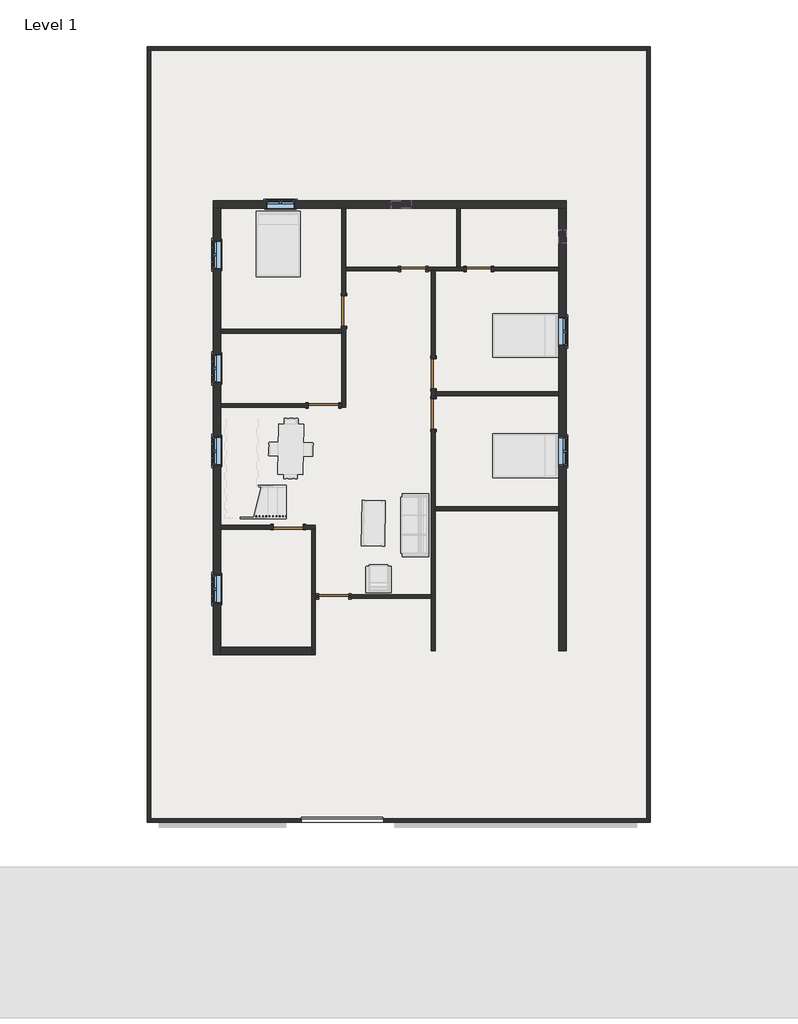
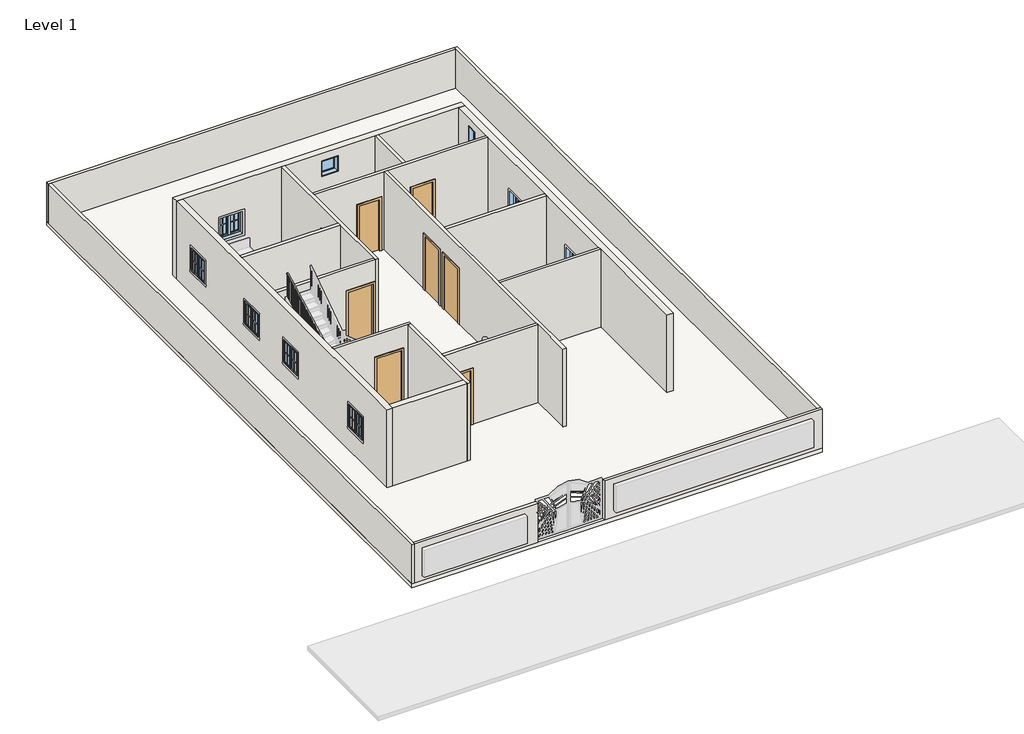
# One storey, part 1 of 2: 20 walls, 9 windows, 8 doors, 1 railing, 1 slab.
"""IFC4 building model written with IfcOpenShell, lengths in millimetres."""

from ifc_helpers import new_model, si_unit, frame, origin, origin_with_axes, place, context, project, spatial, polyline, outline, extrude, faceted_brep, transform, mapped, element, save
from components import door_d8f5dbb5, door_f2b275c1, door_305aa2a5, door_e5f9f3c4, window_aa618e30, window_80340324, window_339605e1

model = new_model("IFC4")

# Units and contexts
model_context = context("Model", 3, world=origin())
ifc_project = project(units=[si_unit("LENGTHUNIT", "METRE", prefix="MILLI")], contexts=[model_context])

# Site, building, storey
site = spatial("IfcSite", under=ifc_project)
building = spatial("IfcBuilding", under=site)
storey = spatial("IfcBuildingStorey", under=building, Name="Level 1", Elevation=0.0)

# Doors
placement = place(None, origin())
door_shape = door_d8f5dbb5(model_context)
element("IfcDoor", 1, ObjectType="Single-Flush : 30\" x 80\"", at=placement, inside=storey, context=model_context, shape_type="MappedRepresentation", body=[
    mapped(door_shape, transform((-551.6099931, 5332.4435985, 0.0), x_axis=(1.0, 0.0, 0.0), y_axis=(0.0, 1.0, 0.0), z_axis=(0.0, 0.0, 1.0))),
])
door_2_shape = door_f2b275c1(model_context)
element("IfcDoor", 2, ObjectType="Single-Flush : 30\" x 80\"", at=placement, inside=storey, context=model_context, shape_type="MappedRepresentation", body=[
    mapped(door_2_shape, transform((1429.5900069, 5332.4435985, 0.0), x_axis=(-1.0, 0.0, 0.0), y_axis=(0.0, -1.0, 0.0), z_axis=(0.0, 0.0, 1.0))),
])
door_3_shape = door_305aa2a5(model_context)
element("IfcDoor", 3, ObjectType="Single-Flush : 36\" x 84\"", at=placement, inside=storey, context=model_context, shape_type="MappedRepresentation", body=[
    mapped(door_3_shape, transform((-2647.1099931, 4062.4435985, 0.0), x_axis=(0.0, -1.0, 0.0), y_axis=(1.0, 0.0, 0.0), z_axis=(0.0, 0.0, 1.0))),
])
element("IfcDoor", 4, ObjectType="Single-Flush : 36\" x 84\"", at=placement, inside=storey, context=model_context, shape_type="MappedRepresentation", body=[
    mapped(door_3_shape, transform((57.9900069, 2170.1435985, 0.0), x_axis=(0.0, -1.0, 0.0), y_axis=(1.0, 0.0, 0.0), z_axis=(0.0, 0.0, 1.0))),
])
element("IfcDoor", 5, ObjectType="Single-Flush : 36\" x 84\"", at=placement, inside=storey, context=model_context, shape_type="MappedRepresentation", body=[
    mapped(door_3_shape, transform((-4323.5099931, -2465.3564015, 0.0), x_axis=(1.0, 0.0, 0.0), y_axis=(0.0, 1.0, 0.0), z_axis=(0.0, 0.0, 1.0))),
])
element("IfcDoor", 6, ObjectType="Single-Flush : 36\" x 84\"", at=placement, inside=storey, context=model_context, shape_type="MappedRepresentation", body=[
    mapped(door_3_shape, transform((-2951.9099931, -4560.8564015, 0.0), x_axis=(-1.0, 0.0, 0.0), y_axis=(0.0, -1.0, 0.0), z_axis=(0.0, 0.0, 1.0))),
])
door_4_shape = door_e5f9f3c4(model_context)
element("IfcDoor", 7, ObjectType="Single-Flush : 36\" x 84\"", at=placement, inside=storey, context=model_context, shape_type="MappedRepresentation", body=[
    mapped(door_4_shape, transform((-3256.7099931, 1204.9435985, 0.0), x_axis=(1.0, 0.0, 0.0), y_axis=(0.0, 1.0, 0.0), z_axis=(0.0, 0.0, 1.0))),
])
element("IfcDoor", 8, ObjectType="Single-Flush : 36\" x 84\"", at=placement, inside=storey, context=model_context, shape_type="MappedRepresentation", body=[
    mapped(door_4_shape, transform((57.9900069, 950.9435985, 0.0), x_axis=(0.0, 1.0, 0.0), y_axis=(-1.0, 0.0, 0.0), z_axis=(0.0, 0.0, 1.0))),
])

# Railing
element("IfcRailing", 9, ObjectType="Handrail - Rectangular", at=placement, inside=storey, context=model_context, shape_type="SolidModel", body=[
    faceted_brep([(-4378.4230036, -2160.5564015, 1761.0666667), (-4378.4230036, -2160.5564015, 1704.9107192), (-4378.4230036, -2109.7564015, 1704.9107192), (-4378.4230036, -2109.7564015, 1761.0666667), (-5973.5005957, -2160.5564015, 2512.5835228), (-5984.8684735, -2160.5564015, 2461.7835228), (-5984.8684735, -2109.7564015, 2461.7835228), (-5973.5005957, -2109.7564015, 2512.5835228), (-6196.7599931, -2160.5564015, 2512.5835228), (-6196.7599931, -2160.5564015, 2461.7835228), (-6145.9599931, -2109.7564015, 2461.7835228), (-6145.9599931, -2109.7564015, 2512.5835228), (-6196.7599931, -1959.3194067, 2512.5835228), (-6196.7599931, -1946.6862419, 2461.7835228), (-6145.9599931, -1946.6862419, 2461.7835228), (-6145.9599931, -1959.3194067, 2512.5835228), (-6196.7599931, 775.380588, 3962.4), (-6145.9599931, 775.380588, 3962.4), (-6145.9599931, 775.380588, 3904.9024571), (-6196.7599931, 775.380588, 3904.9024571)], [[[0, 1, 2, 3]], [[1, 0, 4, 5]], [[2, 1, 5, 6]], [[3, 2, 6, 7]], [[0, 3, 7, 4]], [[5, 4, 8, 9]], [[6, 5, 9, 10]], [[7, 6, 10, 11]], [[4, 7, 11, 8]], [[9, 8, 12, 13]], [[10, 9, 13, 14]], [[11, 10, 14, 15]], [[8, 11, 15, 12]], [[16, 17, 18, 19]], [[13, 12, 16, 19]], [[14, 13, 19, 18]], [[15, 14, 18, 17]], [[12, 15, 17, 16]]]),
    extrude(outline(polyline([(719.1685985, 3875.1013569), (719.1685985, 2878.6666667), (700.1185985, 2878.6666667), (700.1185985, 3865.001893), (719.1685985, 3875.1013569)])), frame((-6180.8849931, 0.0, 0.0), z_axis=(1.0, 0.0, 0.0), x_axis=(0.0, 1.0, 0.0)), (0.0, 0.0, 1.0), 19.05),
    extrude(outline(polyline([(617.5685985, 3821.2375494), (617.5685985, 2878.6666667), (598.5185985, 2878.6666667), (598.5185985, 3811.1380855), (617.5685985, 3821.2375494)])), frame((-6180.8849931, 0.0, 0.0), z_axis=(1.0, 0.0, 0.0), x_axis=(0.0, 1.0, 0.0)), (0.0, 0.0, 1.0), 19.05),
    extrude(outline(polyline([(515.9685985, 3767.3737419), (515.9685985, 2878.6666667), (496.9185985, 2878.6666667), (496.9185985, 3757.274278), (515.9685985, 3767.3737419)])), frame((-6180.8849931, 0.0, 0.0), z_axis=(1.0, 0.0, 0.0), x_axis=(0.0, 1.0, 0.0)), (0.0, 0.0, 1.0), 19.05),
    extrude(outline(polyline([(414.3685985, 3713.5099344), (414.3685985, 2709.3333333), (395.3185985, 2709.3333333), (395.3185985, 3703.4104705), (414.3685985, 3713.5099344)])), frame((-6180.8849931, 0.0, 0.0), z_axis=(1.0, 0.0, 0.0), x_axis=(0.0, 1.0, 0.0)), (0.0, 0.0, 1.0), 19.05),
    extrude(outline(polyline([(312.7685985, 3659.6461269), (312.7685985, 2709.3333333), (293.7185985, 2709.3333333), (293.7185985, 3649.546663), (312.7685985, 3659.6461269)])), frame((-6180.8849931, 0.0, 0.0), z_axis=(1.0, 0.0, 0.0), x_axis=(0.0, 1.0, 0.0)), (0.0, 0.0, 1.0), 19.05),
    extrude(outline(polyline([(211.1685985, 3605.7823194), (211.1685985, 2540.0), (192.1185985, 2540.0), (192.1185985, 3595.6828555), (211.1685985, 3605.7823194)])), frame((-6180.8849931, 0.0, 0.0), z_axis=(1.0, 0.0, 0.0), x_axis=(0.0, 1.0, 0.0)), (0.0, 0.0, 1.0), 19.05),
    extrude(outline(polyline([(109.5685985, 3551.9185119), (109.5685985, 2540.0), (90.5185985, 2540.0), (90.5185985, 3541.819048), (109.5685985, 3551.9185119)])), frame((-6180.8849931, 0.0, 0.0), z_axis=(1.0, 0.0, 0.0), x_axis=(0.0, 1.0, 0.0)), (0.0, 0.0, 1.0), 19.05),
    extrude(outline(polyline([(7.9685985, 3498.0547044), (7.9685985, 2540.0), (-11.0814015, 2540.0), (-11.0814015, 3487.9552405), (7.9685985, 3498.0547044)])), frame((-6180.8849931, 0.0, 0.0), z_axis=(1.0, 0.0, 0.0), x_axis=(0.0, 1.0, 0.0)), (0.0, 0.0, 1.0), 19.05),
    extrude(outline(polyline([(-93.6314015, 3444.1908969), (-93.6314015, 2370.6666667), (-112.6814015, 2370.6666667), (-112.6814015, 3434.091433), (-93.6314015, 3444.1908969)])), frame((-6180.8849931, 0.0, 0.0), z_axis=(1.0, 0.0, 0.0), x_axis=(0.0, 1.0, 0.0)), (0.0, 0.0, 1.0), 19.05),
    extrude(outline(polyline([(-195.2314015, 3390.3270894), (-195.2314015, 2370.6666667), (-214.2814015, 2370.6666667), (-214.2814015, 3380.2276255), (-195.2314015, 3390.3270894)])), frame((-6180.8849931, 0.0, 0.0), z_axis=(1.0, 0.0, 0.0), x_axis=(0.0, 1.0, 0.0)), (0.0, 0.0, 1.0), 19.05),
    extrude(outline(polyline([(-296.8314015, 3336.4632819), (-296.8314015, 2370.6666667), (-315.8814015, 2370.6666667), (-315.8814015, 3326.363818), (-296.8314015, 3336.4632819)])), frame((-6180.8849931, 0.0, 0.0), z_axis=(1.0, 0.0, 0.0), x_axis=(0.0, 1.0, 0.0)), (0.0, 0.0, 1.0), 19.05),
    extrude(outline(polyline([(-398.4314015, 3282.5994744), (-398.4314015, 2201.3333333), (-417.4814015, 2201.3333333), (-417.4814015, 3272.5000105), (-398.4314015, 3282.5994744)])), frame((-6180.8849931, 0.0, 0.0), z_axis=(1.0, 0.0, 0.0), x_axis=(0.0, 1.0, 0.0)), (0.0, 0.0, 1.0), 19.05),
    extrude(outline(polyline([(-500.0314015, 3228.7356669), (-500.0314015, 2201.3333333), (-519.0814015, 2201.3333333), (-519.0814015, 3218.636203), (-500.0314015, 3228.7356669)])), frame((-6180.8849931, 0.0, 0.0), z_axis=(1.0, 0.0, 0.0), x_axis=(0.0, 1.0, 0.0)), (0.0, 0.0, 1.0), 19.05),
    extrude(outline(polyline([(-601.6314015, 3174.8718594), (-601.6314015, 2201.3333333), (-620.6814015, 2201.3333333), (-620.6814015, 3164.7723955), (-601.6314015, 3174.8718594)])), frame((-6180.8849931, 0.0, 0.0), z_axis=(1.0, 0.0, 0.0), x_axis=(0.0, 1.0, 0.0)), (0.0, 0.0, 1.0), 19.05),
    extrude(outline(polyline([(-703.2314015, 3121.0080519), (-703.2314015, 2032.0), (-722.2814015, 2032.0), (-722.2814015, 3110.908588), (-703.2314015, 3121.0080519)])), frame((-6180.8849931, 0.0, 0.0), z_axis=(1.0, 0.0, 0.0), x_axis=(0.0, 1.0, 0.0)), (0.0, 0.0, 1.0), 19.05),
    extrude(outline(polyline([(-804.8314015, 3067.1442444), (-804.8314015, 2032.0), (-823.8814015, 2032.0), (-823.8814015, 3057.0447805), (-804.8314015, 3067.1442444)])), frame((-6180.8849931, 0.0, 0.0), z_axis=(1.0, 0.0, 0.0), x_axis=(0.0, 1.0, 0.0)), (0.0, 0.0, 1.0), 19.05),
    extrude(outline(polyline([(-906.4314015, 3013.2804369), (-906.4314015, 2032.0), (-925.4814015, 2032.0), (-925.4814015, 3003.180973), (-906.4314015, 3013.2804369)])), frame((-6180.8849931, 0.0, 0.0), z_axis=(1.0, 0.0, 0.0), x_axis=(0.0, 1.0, 0.0)), (0.0, 0.0, 1.0), 19.05),
    extrude(outline(polyline([(-1008.0314015, 2959.4166294), (-1008.0314015, 1862.6666667), (-1027.0814015, 1862.6666667), (-1027.0814015, 2949.3171655), (-1008.0314015, 2959.4166294)])), frame((-6180.8849931, 0.0, 0.0), z_axis=(1.0, 0.0, 0.0), x_axis=(0.0, 1.0, 0.0)), (0.0, 0.0, 1.0), 19.05),
    extrude(outline(polyline([(-1109.6314015, 2905.5528219), (-1109.6314015, 1862.6666667), (-1128.6814015, 1862.6666667), (-1128.6814015, 2895.453358), (-1109.6314015, 2905.5528219)])), frame((-6180.8849931, 0.0, 0.0), z_axis=(1.0, 0.0, 0.0), x_axis=(0.0, 1.0, 0.0)), (0.0, 0.0, 1.0), 19.05),
    extrude(outline(polyline([(-1211.2314015, 2851.6890144), (-1211.2314015, 1862.6666667), (-1230.2814015, 1862.6666667), (-1230.2814015, 2841.5895505), (-1211.2314015, 2851.6890144)])), frame((-6180.8849931, 0.0, 0.0), z_axis=(1.0, 0.0, 0.0), x_axis=(0.0, 1.0, 0.0)), (0.0, 0.0, 1.0), 19.05),
    extrude(outline(polyline([(-1312.8314015, 2797.8252069), (-1312.8314015, 1862.6666667), (-1331.8814015, 1862.6666667), (-1331.8814015, 2787.725743), (-1312.8314015, 2797.8252069)])), frame((-6180.8849931, 0.0, 0.0), z_axis=(1.0, 0.0, 0.0), x_axis=(0.0, 1.0, 0.0)), (0.0, 0.0, 1.0), 19.05),
    extrude(outline(polyline([(-1414.4314015, 2743.9613994), (-1414.4314015, 1693.3333333), (-1433.4814015, 1693.3333333), (-1433.4814015, 2733.8619355), (-1414.4314015, 2743.9613994)])), frame((-6180.8849931, 0.0, 0.0), z_axis=(1.0, 0.0, 0.0), x_axis=(0.0, 1.0, 0.0)), (0.0, 0.0, 1.0), 19.05),
    extrude(outline(polyline([(-1516.0314015, 2690.0975919), (-1516.0314015, 1693.3333333), (-1535.0814015, 1693.3333333), (-1535.0814015, 2679.998128), (-1516.0314015, 2690.0975919)])), frame((-6180.8849931, 0.0, 0.0), z_axis=(1.0, 0.0, 0.0), x_axis=(0.0, 1.0, 0.0)), (0.0, 0.0, 1.0), 19.05),
    extrude(outline(polyline([(-1617.6314015, 2636.2337844), (-1617.6314015, 1693.3333333), (-1636.6814015, 1693.3333333), (-1636.6814015, 2626.1343205), (-1617.6314015, 2636.2337844)])), frame((-6180.8849931, 0.0, 0.0), z_axis=(1.0, 0.0, 0.0), x_axis=(0.0, 1.0, 0.0)), (0.0, 0.0, 1.0), 19.05),
    extrude(outline(polyline([(-1719.2314015, 2582.3699769), (-1719.2314015, 1693.3333333), (-1738.2814015, 1693.3333333), (-1738.2814015, 2572.270513), (-1719.2314015, 2582.3699769)])), frame((-6180.8849931, 0.0, 0.0), z_axis=(1.0, 0.0, 0.0), x_axis=(0.0, 1.0, 0.0)), (0.0, 0.0, 1.0), 19.05),
    extrude(outline(polyline([(-1820.8314015, 2528.5061694), (-1820.8314015, 1524.0), (-1839.8814015, 1524.0), (-1839.8814015, 2518.4067055), (-1820.8314015, 2528.5061694)])), frame((-6180.8849931, 0.0, 0.0), z_axis=(1.0, 0.0, 0.0), x_axis=(0.0, 1.0, 0.0)), (0.0, 0.0, 1.0), 19.05),
    extrude(outline(polyline([(-1922.4314015, 2474.6423619), (-1922.4314015, 1524.0), (-1941.4814015, 1524.0), (-1941.4814015, 2464.542898), (-1922.4314015, 2474.6423619)])), frame((-6180.8849931, 0.0, 0.0), z_axis=(1.0, 0.0, 0.0), x_axis=(0.0, 1.0, 0.0)), (0.0, 0.0, 1.0), 19.05),
    extrude(outline(polyline([(-6180.8849931, -2043.0814015), (-6180.8849931, -2024.0314015), (-6161.8349931, -2024.0314015), (-6161.8349931, -2043.0814015), (-6180.8849931, -2043.0814015)])), frame((0.0, 0.0, 1524.0), z_axis=(0.0, 0.0, 1.0), x_axis=(1.0, 0.0, 0.0)), (0.0, 0.0, 1.0), 937.7835228),
    extrude(outline(polyline([(-6096.0980036, -2144.6814015), (-6115.1480036, -2144.6814015), (-6115.1480036, -2125.6314015), (-6096.0980036, -2125.6314015), (-6096.0980036, -2144.6814015)])), frame((0.0, 0.0, 1524.0), z_axis=(0.0, 0.0, 1.0), x_axis=(1.0, 0.0, 0.0)), (0.0, 0.0, 1.0), 937.7835228),
    extrude(outline(polyline([(-5994.4980036, -2144.6814015), (-6013.5480036, -2144.6814015), (-6013.5480036, -2125.6314015), (-5994.4980036, -2125.6314015), (-5994.4980036, -2144.6814015)])), frame((0.0, 0.0, 1524.0), z_axis=(0.0, 0.0, 1.0), x_axis=(1.0, 0.0, 0.0)), (0.0, 0.0, 1.0), 937.7835228),
    extrude(outline(polyline([(2427.427224, -5911.9480036), (1524.0, -5911.9480036), (1524.0, -5892.8980036), (2418.4518637, -5892.8980036), (2427.427224, -5911.9480036)])), frame((0.0, -2144.6814015, 0.0), z_axis=(0.0, 1.0, 0.0), x_axis=(0.0, 0.0, 1.0)), (0.0, 0.0, 1.0), 19.05),
    extrude(outline(polyline([(2379.5586357, -5810.3480036), (1524.0, -5810.3480036), (1524.0, -5791.2980036), (2370.5832754, -5791.2980036), (2379.5586357, -5810.3480036)])), frame((0.0, -2144.6814015, 0.0), z_axis=(0.0, 1.0, 0.0), x_axis=(0.0, 0.0, 1.0)), (0.0, 0.0, 1.0), 19.05),
    extrude(outline(polyline([(2331.6900474, -5708.7480036), (1354.6666667, -5708.7480036), (1354.6666667, -5689.6980036), (2322.7146871, -5689.6980036), (2331.6900474, -5708.7480036)])), frame((0.0, -2144.6814015, 0.0), z_axis=(0.0, 1.0, 0.0), x_axis=(0.0, 0.0, 1.0)), (0.0, 0.0, 1.0), 19.05),
    extrude(outline(polyline([(2283.8214591, -5607.1480036), (1354.6666667, -5607.1480036), (1354.6666667, -5588.0980036), (2274.8460988, -5588.0980036), (2283.8214591, -5607.1480036)])), frame((0.0, -2144.6814015, 0.0), z_axis=(0.0, 1.0, 0.0), x_axis=(0.0, 0.0, 1.0)), (0.0, 0.0, 1.0), 19.05),
    extrude(outline(polyline([(2235.9528708, -5505.5480036), (1354.6666667, -5505.5480036), (1354.6666667, -5486.4980036), (2226.9775105, -5486.4980036), (2235.9528708, -5505.5480036)])), frame((0.0, -2144.6814015, 0.0), z_axis=(0.0, 1.0, 0.0), x_axis=(0.0, 0.0, 1.0)), (0.0, 0.0, 1.0), 19.05),
    extrude(outline(polyline([(2188.0842825, -5403.9480036), (1354.6666667, -5403.9480036), (1354.6666667, -5384.8980036), (2179.1089222, -5384.8980036), (2188.0842825, -5403.9480036)])), frame((0.0, -2144.6814015, 0.0), z_axis=(0.0, 1.0, 0.0), x_axis=(0.0, 0.0, 1.0)), (0.0, 0.0, 1.0), 19.05),
    extrude(outline(polyline([(2140.2156942, -5302.3480036), (1185.3333333, -5302.3480036), (1185.3333333, -5283.2980036), (2131.2403338, -5283.2980036), (2140.2156942, -5302.3480036)])), frame((0.0, -2144.6814015, 0.0), z_axis=(0.0, 1.0, 0.0), x_axis=(0.0, 0.0, 1.0)), (0.0, 0.0, 1.0), 19.05),
    extrude(outline(polyline([(2092.3471058, -5200.7480036), (1185.3333333, -5200.7480036), (1185.3333333, -5181.6980036), (2083.3717455, -5181.6980036), (2092.3471058, -5200.7480036)])), frame((0.0, -2144.6814015, 0.0), z_axis=(0.0, 1.0, 0.0), x_axis=(0.0, 0.0, 1.0)), (0.0, 0.0, 1.0), 19.05),
    extrude(outline(polyline([(2044.4785175, -5099.1480036), (1185.3333333, -5099.1480036), (1185.3333333, -5080.0980036), (2035.5031572, -5080.0980036), (2044.4785175, -5099.1480036)])), frame((0.0, -2144.6814015, 0.0), z_axis=(0.0, 1.0, 0.0), x_axis=(0.0, 0.0, 1.0)), (0.0, 0.0, 1.0), 19.05),
    extrude(outline(polyline([(1996.6099292, -4997.5480036), (1185.3333333, -4997.5480036), (1185.3333333, -4978.4980036), (1987.6345689, -4978.4980036), (1996.6099292, -4997.5480036)])), frame((0.0, -2144.6814015, 0.0), z_axis=(0.0, 1.0, 0.0), x_axis=(0.0, 0.0, 1.0)), (0.0, 0.0, 1.0), 19.05),
    extrude(outline(polyline([(1948.7413409, -4895.9480036), (1016.0, -4895.9480036), (1016.0, -4876.8980036), (1939.7659806, -4876.8980036), (1948.7413409, -4895.9480036)])), frame((0.0, -2144.6814015, 0.0), z_axis=(0.0, 1.0, 0.0), x_axis=(0.0, 0.0, 1.0)), (0.0, 0.0, 1.0), 19.05),
    extrude(outline(polyline([(1900.8727526, -4794.3480036), (1016.0, -4794.3480036), (1016.0, -4775.2980036), (1891.8973923, -4775.2980036), (1900.8727526, -4794.3480036)])), frame((0.0, -2144.6814015, 0.0), z_axis=(0.0, 1.0, 0.0), x_axis=(0.0, 0.0, 1.0)), (0.0, 0.0, 1.0), 19.05),
    extrude(outline(polyline([(1853.0041643, -4692.7480036), (1016.0, -4692.7480036), (1016.0, -4673.6980036), (1844.028804, -4673.6980036), (1853.0041643, -4692.7480036)])), frame((0.0, -2144.6814015, 0.0), z_axis=(0.0, 1.0, 0.0), x_axis=(0.0, 0.0, 1.0)), (0.0, 0.0, 1.0), 19.05),
    extrude(outline(polyline([(1805.135576, -4591.1480036), (846.6666667, -4591.1480036), (846.6666667, -4572.0980036), (1796.1602157, -4572.0980036), (1805.135576, -4591.1480036)])), frame((0.0, -2144.6814015, 0.0), z_axis=(0.0, 1.0, 0.0), x_axis=(0.0, 0.0, 1.0)), (0.0, 0.0, 1.0), 19.05),
    extrude(outline(polyline([(1757.2669877, -4489.5480036), (846.6666667, -4489.5480036), (846.6666667, -4470.4980036), (1748.2916274, -4470.4980036), (1757.2669877, -4489.5480036)])), frame((0.0, -2144.6814015, 0.0), z_axis=(0.0, 1.0, 0.0), x_axis=(0.0, 0.0, 1.0)), (0.0, 0.0, 1.0), 19.05),
    extrude(outline(polyline([(-6161.8349931, -2144.6814015), (-6180.8849931, -2144.6814015), (-6180.8849931, -2125.6314015), (-6161.8349931, -2125.6314015), (-6161.8349931, -2144.6814015)])), frame((0.0, 0.0, 1524.0), z_axis=(0.0, 0.0, 1.0), x_axis=(1.0, 0.0, 0.0)), (0.0, 0.0, 1.0), 937.7835228),
    extrude(outline(polyline([(775.380588, 3904.9024571), (775.380588, 2878.6666667), (756.330588, 2878.6666667), (756.330588, 3894.8029932), (775.380588, 3904.9024571)])), frame((-6180.8849931, 0.0, 0.0), z_axis=(1.0, 0.0, 0.0), x_axis=(0.0, 1.0, 0.0)), (0.0, 0.0, 1.0), 19.05),
    extrude(outline(polyline([(1713.8860795, -4397.4730036), (846.6666667, -4397.4730036), (846.6666667, -4378.4230036), (1704.9107192, -4378.4230036), (1713.8860795, -4397.4730036)])), frame((0.0, -2144.6814015, 0.0), z_axis=(0.0, 1.0, 0.0), x_axis=(0.0, 0.0, 1.0)), (0.0, 0.0, 1.0), 19.05),
])

# Slab
element("IfcSlab", 10, ObjectType="Generic - 12\"", at=placement, inside=storey, context=model_context, shape_type="SweptSolid", body=[
    extrude(outline(polyline([(6616.5772651, 12050.2767292), (6616.5772651, -11381.2232708), (-8585.3227349, -11381.2232708), (-8585.3227349, 12050.2767292), (6616.5772651, 12050.2767292)])), frame((0.0, 0.0, -152.4), z_axis=(0.0, 0.0, 1.0), x_axis=(1.0, 0.0, 0.0)), (0.0, 0.0, 1.0), 152.4),
])

# Walls
element("IfcWall", 11, ObjectType="WALL4.5\"", at=placement, inside=storey, context=model_context, shape_type="SweptSolid", body=[
    extrude(outline(polyline([(-2704.2599931, 3395.6935985), (-6361.8599931, 3395.6935985), (-6361.8599931, 3509.9935985), (-2704.2599931, 3509.9935985), (-2704.2599931, 3395.6935985)])), origin_with_axes(), (0.0, 0.0, 1.0), 3048.0),
])
element("IfcWall", 12, ObjectType="WALL4.5\"", at=placement, inside=storey, context=model_context, shape_type="Brep", body=[
    faceted_brep([(-2704.2599931, 3605.2435985, 2133.6), (-2704.2599931, 3605.2435985, 0.0), (-2704.2599931, 3509.9935985, 0.0), (-2704.2599931, 3395.6935985, 0.0), (-2704.2599931, 1262.0935985, 0.0), (-2704.2599931, 1147.7935985, 0.0), (-2704.2599931, 1147.7935985, 3048.0), (-2704.2599931, 1262.0935985, 3048.0), (-2704.2599931, 3395.6935985, 3048.0), (-2704.2599931, 3509.9935985, 3048.0), (-2704.2599931, 7167.5935985, 3048.0), (-2704.2599931, 7167.5935985, 0.0), (-2704.2599931, 4519.6435985, 0.0), (-2704.2599931, 4519.6435985, 2133.6), (-2589.9599931, 1147.7935985, 0.0), (-2589.9599931, 3605.2435985, 0.0), (-2589.9599931, 3605.2435985, 2133.6), (-2589.9599931, 4519.6435985, 2133.6), (-2589.9599931, 4519.6435985, 0.0), (-2589.9599931, 5275.2935985, 0.0), (-2589.9599931, 5389.5935985, 0.0), (-2589.9599931, 7167.5935985, 0.0), (-2589.9599931, 7167.5935985, 3048.0), (-2589.9599931, 5389.5935985, 3048.0), (-2589.9599931, 5275.2935985, 3048.0), (-2589.9599931, 1147.7935985, 3048.0)], [[[0, 1, 2, 3, 4, 5, 6, 7, 8, 9, 10, 11, 12, 13]], [[14, 15, 16, 17, 18, 19, 20, 21, 22, 23, 24, 25]], [[12, 11, 21, 20, 19, 18]], [[5, 4, 3, 2, 1, 15, 14]], [[11, 10, 22, 21]], [[6, 5, 14, 25]], [[16, 15, 1, 0]], [[17, 16, 0, 13]], [[18, 17, 13, 12]], [[10, 9, 8, 7, 6, 25, 24, 23, 22]]]),
])
element("IfcWall", 13, ObjectType="WALL4.5\"", at=placement, inside=storey, context=model_context, shape_type="SweptSolid", body=[
    extrude(outline(polyline([(2133.6, -2799.5099931), (0.0, -2799.5099931), (0.0, -2704.2599931), (3048.0, -2704.2599931), (3048.0, -6361.8599931), (0.0, -6361.8599931), (0.0, -3713.9099931), (2133.6, -3713.9099931), (2133.6, -2799.5099931)])), frame((0.0, 1147.7935985, 0.0), z_axis=(0.0, 1.0, 0.0), x_axis=(0.0, 0.0, 1.0)), (0.0, 0.0, 1.0), 114.3),
])
element("IfcWall", 14, ObjectType="WALL4.5\"", at=placement, inside=storey, context=model_context, shape_type="Brep", body=[
    faceted_brep([(-170.6099931, 5275.2935985, 0.0), (0.8400069, 5275.2935985, 0.0), (115.1400069, 5275.2935985, 0.0), (1048.5900069, 5275.2935985, 0.0), (1048.5900069, 5275.2935985, 2032.0), (1810.5900069, 5275.2935985, 2032.0), (1810.5900069, 5275.2935985, 0.0), (3848.9400069, 5275.2935985, 0.0), (3848.9400069, 5275.2935985, 3048.0), (115.1400069, 5275.2935985, 3048.0), (0.8400069, 5275.2935985, 3048.0), (-2589.9599931, 5275.2935985, 3048.0), (-2589.9599931, 5275.2935985, 0.0), (-932.6099931, 5275.2935985, 0.0), (-932.6099931, 5275.2935985, 2032.0), (-170.6099931, 5275.2935985, 2032.0), (1048.5900069, 5389.5935985, 2032.0), (1048.5900069, 5389.5935985, 0.0), (877.1400069, 5389.5935985, 0.0), (762.8400069, 5389.5935985, 0.0), (-170.6099931, 5389.5935985, 0.0), (-170.6099931, 5389.5935985, 2032.0), (-932.6099931, 5389.5935985, 2032.0), (-932.6099931, 5389.5935985, 0.0), (-2589.9599931, 5389.5935985, 0.0), (-2589.9599931, 5389.5935985, 3048.0), (762.8400069, 5389.5935985, 3048.0), (877.1400069, 5389.5935985, 3048.0), (3848.9400069, 5389.5935985, 3048.0), (3848.9400069, 5389.5935985, 0.0), (1810.5900069, 5389.5935985, 0.0), (1810.5900069, 5389.5935985, 2032.0)], [[[0, 1, 2, 3, 4, 5, 6, 7, 8, 9, 10, 11, 12, 13, 14, 15]], [[16, 17, 18, 19, 20, 21, 22, 23, 24, 25, 26, 27, 28, 29, 30, 31]], [[13, 12, 24, 23]], [[30, 29, 7, 6]], [[20, 19, 18, 17, 3, 2, 1, 0]], [[8, 7, 29, 28]], [[12, 11, 25, 24]], [[21, 20, 0, 15]], [[22, 21, 15, 14]], [[23, 22, 14, 13]], [[4, 3, 17, 16]], [[5, 4, 16, 31]], [[6, 5, 31, 30]], [[11, 10, 9, 8, 28, 27, 26, 25]]]),
])
element("IfcWall", 15, ObjectType="WALL4.5\"", at=placement, inside=storey, context=model_context, shape_type="SweptSolid", body=[
    extrude(outline(polyline([(762.8400069, 5389.5935985), (762.8400069, 7167.5935985), (877.1400069, 7167.5935985), (877.1400069, 5389.5935985), (762.8400069, 5389.5935985)])), origin_with_axes(), (0.0, 0.0, 1.0), 3048.0),
])
element("IfcWall", 16, ObjectType="WALL4.5\"", at=placement, inside=storey, context=model_context, shape_type="Brep", body=[
    faceted_brep([(0.8400069, 1712.9435985, 0.0), (0.8400069, 1408.1435985, 0.0), (0.8400069, 1408.1435985, 2133.6), (0.8400069, 493.7435985, 2133.6), (0.8400069, 493.7435985, 0.0), (0.8400069, -4503.7064015, 0.0), (0.8400069, -4618.0064015, 0.0), (0.8400069, -6205.5064015, 0.0), (0.8400069, -6205.5064015, 3048.0), (0.8400069, -4618.0064015, 3048.0), (0.8400069, -4503.7064015, 3048.0), (0.8400069, 5275.2935985, 3048.0), (0.8400069, 5275.2935985, 0.0), (0.8400069, 2627.3435985, 0.0), (0.8400069, 2627.3435985, 2133.6), (0.8400069, 1712.9435985, 2133.6), (115.1400069, 1408.1435985, 2133.6), (115.1400069, 1408.1435985, 0.0), (115.1400069, 1503.3935985, 0.0), (115.1400069, 1617.6935985, 0.0), (115.1400069, 1712.9435985, 0.0), (115.1400069, 1712.9435985, 2133.6), (115.1400069, 2627.3435985, 2133.6), (115.1400069, 2627.3435985, 0.0), (115.1400069, 5275.2935985, 0.0), (115.1400069, 5275.2935985, 3048.0), (115.1400069, 1617.6935985, 3048.0), (115.1400069, 1503.3935985, 3048.0), (115.1400069, -1850.058017, 3048.0), (115.1400069, -1964.358017, 3048.0), (115.1400069, -6205.5064015, 3048.0), (115.1400069, -6205.5064015, 0.0), (115.1400069, -1964.358017, 0.0), (115.1400069, -1850.058017, 0.0), (115.1400069, 493.7435985, 0.0), (115.1400069, 493.7435985, 2133.6)], [[[0, 1, 2, 3, 4, 5, 6, 7, 8, 9, 10, 11, 12, 13, 14, 15]], [[16, 17, 18, 19, 20, 21, 22, 23, 24, 25, 26, 27, 28, 29, 30, 31, 32, 33, 34, 35]], [[13, 12, 24, 23]], [[34, 33, 32, 31, 7, 6, 5, 4]], [[20, 19, 18, 17, 1, 0]], [[8, 7, 31, 30]], [[12, 11, 25, 24]], [[21, 20, 0, 15]], [[22, 21, 15, 14]], [[23, 22, 14, 13]], [[2, 1, 17, 16]], [[3, 2, 16, 35]], [[4, 3, 35, 34]], [[11, 10, 9, 8, 30, 29, 28, 27, 26, 25]]]),
])
element("IfcWall", 17, ObjectType="WALL4.5\"", at=placement, inside=storey, context=model_context, shape_type="SweptSolid", body=[
    extrude(outline(polyline([(3848.9400069, -1964.358017), (115.1400069, -1964.358017), (115.1400069, -1850.058017), (3848.9400069, -1850.058017), (3848.9400069, -1964.358017)])), origin_with_axes(), (0.0, 0.0, 1.0), 3048.0),
])
element("IfcWall", 18, ObjectType="WALL4.5\"", at=placement, inside=storey, context=model_context, shape_type="SweptSolid", body=[
    extrude(outline(polyline([(3848.9400069, 1503.3935985), (115.1400069, 1503.3935985), (115.1400069, 1617.6935985), (3848.9400069, 1617.6935985), (3848.9400069, 1503.3935985)])), origin_with_axes(), (0.0, 0.0, 1.0), 3048.0),
])
element("IfcWall", 19, ObjectType="WALL4.5\"", at=placement, inside=storey, context=model_context, shape_type="Brep", body=[
    faceted_brep([(-3866.3099931, -2522.5064015, 2133.6), (-3866.3099931, -2522.5064015, 0.0), (-3618.6599931, -2522.5064015, 0.0), (-3504.3599931, -2522.5064015, 0.0), (-3504.3599931, -2522.5064015, 3048.0), (-3618.6599931, -2522.5064015, 3048.0), (-6361.8599931, -2522.5064015, 3048.0), (-6361.8599931, -2522.5064015, 0.0), (-4780.7099931, -2522.5064015, 0.0), (-4780.7099931, -2522.5064015, 2133.6), (-3504.3599931, -2408.2064015, 0.0), (-3866.3099931, -2408.2064015, 0.0), (-3866.3099931, -2408.2064015, 2133.6), (-4780.7099931, -2408.2064015, 2133.6), (-4780.7099931, -2408.2064015, 0.0), (-6361.8599931, -2408.2064015, 0.0), (-6361.8599931, -2408.2064015, 3048.0), (-3504.3599931, -2408.2064015, 3048.0)], [[[0, 1, 2, 3, 4, 5, 6, 7, 8, 9]], [[10, 11, 12, 13, 14, 15, 16, 17]], [[8, 7, 15, 14]], [[3, 2, 1, 11, 10]], [[7, 6, 16, 15]], [[4, 3, 10, 17]], [[12, 11, 1, 0]], [[13, 12, 0, 9]], [[14, 13, 9, 8]], [[6, 5, 4, 17, 16]]]),
])
element("IfcWall", 20, ObjectType="WALL4.5\"", at=placement, inside=storey, context=model_context, shape_type="SweptSolid", body=[
    extrude(outline(polyline([(0.0, -3504.3599931), (0.0, -3409.1099931), (2133.6, -3409.1099931), (2133.6, -2494.7099931), (0.0, -2494.7099931), (0.0, 0.8400069), (3048.0, 0.8400069), (3048.0, -3504.3599931), (0.0, -3504.3599931)])), frame((0.0, -4618.0064015, 0.0), z_axis=(0.0, 1.0, 0.0), x_axis=(0.0, 0.0, 1.0)), (0.0, 0.0, 1.0), 114.3),
])
element("IfcWall", 21, ObjectType="WALL4.5\"", at=placement, inside=storey, context=model_context, shape_type="Brep", body=[
    faceted_brep([(-3504.3599931, -6319.8064015, 0.0), (-3504.3599931, -4618.0064015, 0.0), (-3504.3599931, -4503.7064015, 0.0), (-3504.3599931, -2522.5064015, 0.0), (-3504.3599931, -2522.5064015, 3048.0), (-3504.3599931, -4503.7064015, 3048.0), (-3504.3599931, -4618.0064015, 3048.0), (-3504.3599931, -6319.8064015, 3048.0), (-3618.6599931, -6319.8064015, 0.0), (-3618.6599931, -6319.8064015, 3048.0), (-3618.6599931, -6091.2064015, 3048.0), (-3618.6599931, -2522.5064015, 3048.0), (-3618.6599931, -2522.5064015, 0.0), (-3618.6599931, -6091.2064015, 0.0)], [[[0, 1, 2, 3, 4, 5, 6, 7]], [[8, 9, 10, 11, 12, 13]], [[3, 2, 1, 0, 8, 13, 12]], [[4, 3, 12, 11]], [[7, 6, 5, 4, 11, 10, 9]], [[0, 7, 9, 8]]]),
])
element("IfcWall", 22, ObjectType="WALL4.5\"", at=placement, inside=storey, context=model_context, shape_type="Brep", body=[
    faceted_brep([(-8585.3227349, 11935.9767292, 0.0), (-8471.0227349, 11935.9767292, 0.0), (6502.2772651, 11935.9767292, 0.0), (6502.2772651, 11935.9767292, 1524.0), (-8471.0227349, 11935.9767292, 1524.0), (-8585.3227349, 11935.9767292, 1524.0), (-8585.3227349, 12050.2767292, 0.0), (-8585.3227349, 12050.2767292, 1524.0), (6502.2772651, 12050.2767292, 1524.0), (6502.2772651, 12050.2767292, 0.0)], [[[0, 1, 2, 3, 4, 5]], [[6, 7, 8, 9]], [[2, 1, 0, 6, 9]], [[5, 4, 3, 8, 7]], [[0, 5, 7, 6]], [[3, 2, 9, 8]]]),
])
element("IfcWall", 23, ObjectType="WALL4.5\"", at=placement, inside=storey, context=model_context, shape_type="Brep", body=[
    faceted_brep([(-8471.0227349, -11381.2232708, 0.0), (-8471.0227349, -11266.9232708, 0.0), (-8471.0227349, 11935.9767292, 0.0), (-8471.0227349, 11935.9767292, 1524.0), (-8471.0227349, -11266.9232708, 1524.0), (-8471.0227349, -11381.2232708, 1524.0), (-8585.3227349, -11381.2232708, 0.0), (-8585.3227349, -11381.2232708, 1524.0), (-8585.3227349, 11935.9767292, 1524.0), (-8585.3227349, 11935.9767292, 0.0)], [[[0, 1, 2, 3, 4, 5]], [[6, 7, 8, 9]], [[2, 1, 0, 6, 9]], [[5, 4, 3, 8, 7]], [[0, 5, 7, 6]], [[3, 2, 9, 8]]]),
])
element("IfcWall", 24, ObjectType="WALL4.5\"", at=placement, inside=storey, context=model_context, shape_type="Brep", body=[
    faceted_brep([(6616.5772651, -11266.9232708, 0.0), (6502.2772651, -11266.9232708, 0.0), (-1441.5727349, -11266.9232708, 0.0), (-1441.5727349, -11266.9232708, 1524.0), (6502.2772651, -11266.9232708, 1524.0), (6616.5772651, -11266.9232708, 1524.0), (6616.5772651, -11381.2232708, 0.0), (6616.5772651, -11381.2232708, 1524.0), (-1441.5727349, -11381.2232708, 1524.0), (-1441.5727349, -11381.2232708, 0.0)], [[[0, 1, 2, 3, 4, 5]], [[6, 7, 8, 9]], [[2, 1, 0, 6, 9]], [[3, 2, 9, 8]], [[5, 4, 3, 8, 7]], [[0, 5, 7, 6]]]),
])
element("IfcWall", 25, ObjectType="WALL4.5\"", at=placement, inside=storey, context=model_context, shape_type="Brep", body=[
    faceted_brep([(6502.2772651, 12050.2767292, 0.0), (6502.2772651, 11935.9767292, 0.0), (6502.2772651, -11266.9232708, 0.0), (6502.2772651, -11266.9232708, 1524.0), (6502.2772651, 11935.9767292, 1524.0), (6502.2772651, 12050.2767292, 1524.0), (6616.5772651, 12050.2767292, 0.0), (6616.5772651, 12050.2767292, 1524.0), (6616.5772651, -11266.9232708, 1524.0), (6616.5772651, -11266.9232708, 0.0)], [[[0, 1, 2, 3, 4, 5]], [[6, 7, 8, 9]], [[2, 1, 0, 6, 9]], [[5, 4, 3, 8, 7]], [[0, 5, 7, 6]], [[3, 2, 9, 8]]]),
])
element("IfcWall", 26, ObjectType="WALL4.5\"", at=placement, inside=storey, context=model_context, shape_type="SweptSolid", body=[
    extrude(outline(polyline([(-8471.0227349, -11266.9232708), (-3930.7727349, -11266.9232708), (-3930.7727349, -11381.2232708), (-8471.0227349, -11381.2232708), (-8471.0227349, -11266.9232708)])), origin_with_axes(), (0.0, 0.0, 1.0), 1524.0),
])
element("IfcWall", 27, ObjectType="WALL9\"", at=placement, inside=storey, context=model_context, shape_type="Brep", body=[
    faceted_brep([(-6590.4599931, 7167.5935985, 0.0), (-6361.8599931, 7167.5935985, 0.0), (-2704.2599931, 7167.5935985, 0.0), (-2589.9599931, 7167.5935985, 0.0), (762.8400069, 7167.5935985, 0.0), (877.1400069, 7167.5935985, 0.0), (3848.9400069, 7167.5935985, 0.0), (4077.5400069, 7167.5935985, 0.0), (4077.5400069, 7167.5935985, 3048.0), (3848.9400069, 7167.5935985, 3048.0), (877.1400069, 7167.5935985, 3048.0), (762.8400069, 7167.5935985, 3048.0), (-2589.9599931, 7167.5935985, 3048.0), (-2704.2599931, 7167.5935985, 3048.0), (-6361.8599931, 7167.5935985, 3048.0), (-6590.4599931, 7167.5935985, 3048.0), (-608.7599931, 7167.5935985, 2743.2), (-608.7599931, 7167.5935985, 2133.6), (-1218.3599931, 7167.5935985, 2133.6), (-1218.3599931, 7167.5935985, 2743.2), (-4129.8349931, 7167.5935985, 1828.8), (-4129.8349931, 7167.5935985, 914.4), (-4993.4349931, 7167.5935985, 914.4), (-4993.4349931, 7167.5935985, 1828.8), (4077.5400069, 7396.1935985, 0.0), (-6590.4599931, 7396.1935985, 0.0), (-6590.4599931, 7396.1935985, 3048.0), (4077.5400069, 7396.1935985, 3048.0), (-608.7599931, 7396.1935985, 2133.6), (-608.7599931, 7396.1935985, 2743.2), (-1218.3599931, 7396.1935985, 2743.2), (-1218.3599931, 7396.1935985, 2133.6), (-4129.8349931, 7396.1935985, 914.4), (-4129.8349931, 7396.1935985, 1828.8), (-4993.4349931, 7396.1935985, 1828.8), (-4993.4349931, 7396.1935985, 914.4)], [[[0, 1, 2, 3, 4, 5, 6, 7, 8, 9, 10, 11, 12, 13, 14, 15], [16, 17, 18, 19], [20, 21, 22, 23]], [[24, 25, 26, 27], [28, 29, 30, 31], [32, 33, 34, 35]], [[7, 6, 5, 4, 3, 2, 1, 0, 25, 24]], [[8, 7, 24, 27]], [[0, 15, 26, 25]], [[16, 29, 28, 17]], [[17, 28, 31, 18]], [[18, 31, 30, 19]], [[21, 20, 33, 32]], [[22, 21, 32, 35]], [[23, 22, 35, 34]], [[20, 23, 34, 33]], [[15, 14, 13, 12, 11, 10, 9, 8, 27, 26]], [[29, 16, 19, 30]]]),
])
element("IfcWall", 28, ObjectType="WALL9\"", at=placement, inside=storey, context=model_context, shape_type="Brep", body=[
    faceted_brep([(3848.9400069, 7167.5935985, 0.0), (3848.9400069, 5389.5935985, 0.0), (3848.9400069, 5275.2935985, 0.0), (3848.9400069, 1617.6935985, 0.0), (3848.9400069, 1503.3935985, 0.0), (3848.9400069, -1850.058017, 0.0), (3848.9400069, -1964.358017, 0.0), (3848.9400069, -6205.5064015, 0.0), (3848.9400069, -6205.5064015, 3048.0), (3848.9400069, -1964.358017, 3048.0), (3848.9400069, -1850.058017, 3048.0), (3848.9400069, 1503.3935985, 3048.0), (3848.9400069, 1617.6935985, 3048.0), (3848.9400069, 5275.2935985, 3048.0), (3848.9400069, 5389.5935985, 3048.0), (3848.9400069, 7167.5935985, 3048.0), (3848.9400069, 6103.9685985, 2743.2), (3848.9400069, 6103.9685985, 2133.6), (3848.9400069, 6510.3685985, 2133.6), (3848.9400069, 6510.3685985, 2743.2), (3848.9400069, 3014.6935985, 1828.8), (3848.9400069, 3014.6935985, 914.4), (3848.9400069, 3878.2935985, 914.4), (3848.9400069, 3878.2935985, 1828.8), (3848.9400069, -605.1322092, 1828.8), (3848.9400069, -605.1322092, 914.4), (3848.9400069, 258.4677908, 914.4), (3848.9400069, 258.4677908, 1828.8), (4077.5400069, -6205.5064015, 0.0), (4077.5400069, 7167.5935985, 0.0), (4077.5400069, 7167.5935985, 3048.0), (4077.5400069, -6205.5064015, 3048.0), (4077.5400069, 6103.9685985, 2133.6), (4077.5400069, 6103.9685985, 2743.2), (4077.5400069, 6510.3685985, 2743.2), (4077.5400069, 6510.3685985, 2133.6), (4077.5400069, 3014.6935985, 914.4), (4077.5400069, 3014.6935985, 1828.8), (4077.5400069, 3878.2935985, 1828.8), (4077.5400069, 3878.2935985, 914.4), (4077.5400069, -605.1322092, 914.4), (4077.5400069, -605.1322092, 1828.8), (4077.5400069, 258.4677908, 1828.8), (4077.5400069, 258.4677908, 914.4)], [[[0, 1, 2, 3, 4, 5, 6, 7, 8, 9, 10, 11, 12, 13, 14, 15], [16, 17, 18, 19], [20, 21, 22, 23], [24, 25, 26, 27]], [[28, 29, 30, 31], [32, 33, 34, 35], [36, 37, 38, 39], [40, 41, 42, 43]], [[7, 6, 5, 4, 3, 2, 1, 0, 29, 28]], [[8, 7, 28, 31]], [[0, 15, 30, 29]], [[16, 33, 32, 17]], [[17, 32, 35, 18]], [[18, 35, 34, 19]], [[21, 20, 37, 36]], [[22, 21, 36, 39]], [[23, 22, 39, 38]], [[20, 23, 38, 37]], [[25, 24, 41, 40]], [[26, 25, 40, 43]], [[27, 26, 43, 42]], [[24, 27, 42, 41]], [[15, 14, 13, 12, 11, 10, 9, 8, 31, 30]], [[33, 16, 19, 34]]]),
])
element("IfcWall", 29, ObjectType="WALL9\"", at=placement, inside=storey, context=model_context, shape_type="Brep", body=[
    faceted_brep([(-6361.8599931, -6319.8064015, 0.0), (-6361.8599931, -6091.2064015, 0.0), (-6361.8599931, -2522.5064015, 0.0), (-6361.8599931, -2408.2064015, 0.0), (-6361.8599931, 1147.7935985, 0.0), (-6361.8599931, 1262.0935985, 0.0), (-6361.8599931, 3395.6935985, 0.0), (-6361.8599931, 3509.9935985, 0.0), (-6361.8599931, 7167.5935985, 0.0), (-6361.8599931, 7167.5935985, 3048.0), (-6361.8599931, 3509.9935985, 3048.0), (-6361.8599931, 3395.6935985, 3048.0), (-6361.8599931, 1262.0935985, 3048.0), (-6361.8599931, 1147.7935985, 3048.0), (-6361.8599931, -2408.2064015, 3048.0), (-6361.8599931, -2522.5064015, 3048.0), (-6361.8599931, -6091.2064015, 3048.0), (-6361.8599931, -6319.8064015, 3048.0), (-6361.8599931, 2760.6935985, 1828.8), (-6361.8599931, 2760.6935985, 914.4), (-6361.8599931, 1897.0935985, 914.4), (-6361.8599931, 1897.0935985, 1828.8), (-6361.8599931, 6189.6935985, 1828.8), (-6361.8599931, 6189.6935985, 914.4), (-6361.8599931, 5326.0935985, 914.4), (-6361.8599931, 5326.0935985, 1828.8), (-6361.8599931, -3903.6314015, 1828.8), (-6361.8599931, -3903.6314015, 914.4), (-6361.8599931, -4767.2314015, 914.4), (-6361.8599931, -4767.2314015, 1828.8), (-6361.8599931, 265.1435985, 1828.8), (-6361.8599931, 265.1435985, 914.4), (-6361.8599931, -598.4564015, 914.4), (-6361.8599931, -598.4564015, 1828.8), (-6590.4599931, -6319.8064015, 0.0), (-6590.4599931, -6319.8064015, 3048.0), (-6590.4599931, 7167.5935985, 3048.0), (-6590.4599931, 7167.5935985, 0.0), (-6590.4599931, 2760.6935985, 1828.8), (-6590.4599931, 1897.0935985, 1828.8), (-6590.4599931, 1897.0935985, 914.4), (-6590.4599931, 2760.6935985, 914.4), (-6590.4599931, 6189.6935985, 1828.8), (-6590.4599931, 5326.0935985, 1828.8), (-6590.4599931, 5326.0935985, 914.4), (-6590.4599931, 6189.6935985, 914.4), (-6590.4599931, -3903.6314015, 1828.8), (-6590.4599931, -4767.2314015, 1828.8), (-6590.4599931, -4767.2314015, 914.4), (-6590.4599931, -3903.6314015, 914.4), (-6590.4599931, 265.1435985, 1828.8), (-6590.4599931, -598.4564015, 1828.8), (-6590.4599931, -598.4564015, 914.4), (-6590.4599931, 265.1435985, 914.4)], [[[0, 1, 2, 3, 4, 5, 6, 7, 8, 9, 10, 11, 12, 13, 14, 15, 16, 17], [18, 19, 20, 21], [22, 23, 24, 25], [26, 27, 28, 29], [30, 31, 32, 33]], [[34, 35, 36, 37], [38, 39, 40, 41], [42, 43, 44, 45], [46, 47, 48, 49], [50, 51, 52, 53]], [[8, 7, 6, 5, 4, 3, 2, 1, 0, 34, 37]], [[9, 8, 37, 36]], [[19, 18, 38, 41]], [[20, 19, 41, 40]], [[21, 20, 40, 39]], [[18, 21, 39, 38]], [[23, 22, 42, 45]], [[24, 23, 45, 44]], [[25, 24, 44, 43]], [[22, 25, 43, 42]], [[27, 26, 46, 49]], [[28, 27, 49, 48]], [[29, 28, 48, 47]], [[26, 29, 47, 46]], [[31, 30, 50, 53]], [[32, 31, 53, 52]], [[33, 32, 52, 51]], [[30, 33, 51, 50]], [[17, 16, 15, 14, 13, 12, 11, 10, 9, 36, 35]], [[0, 17, 35, 34]]]),
])
element("IfcWall", 30, ObjectType="WALL9\"", at=placement, inside=storey, context=model_context, shape_type="SweptSolid", body=[
    extrude(outline(polyline([(-3618.6599931, -6319.8064015), (-6361.8599931, -6319.8064015), (-6361.8599931, -6091.2064015), (-3618.6599931, -6091.2064015), (-3618.6599931, -6319.8064015)])), origin_with_axes(), (0.0, 0.0, 1.0), 3048.0),
])

# Windows
window_shape = window_aa618e30(model_context)
element("IfcWindow", 31, ObjectType="Fixed : 16\" x 24\"", at=placement, inside=storey, context=model_context, shape_type="MappedRepresentation", body=[
    mapped(window_shape, transform((3963.2400069, 6269.0685985, 1219.2), x_axis=(0.0, -1.0, 0.0), y_axis=(1.0, 0.0, 0.0), z_axis=(0.0, 0.0, 1.0))),
])
window_2_shape = window_80340324(model_context)
element("IfcWindow", 32, ObjectType="Fixed : 24\" x 24\"", at=placement, inside=storey, context=model_context, shape_type="MappedRepresentation", body=[
    mapped(window_2_shape, transform((-875.4599931, 7281.8935985, 1219.2), x_axis=(1.0, 0.0, 0.0), y_axis=(0.0, 1.0, 0.0), z_axis=(0.0, 0.0, 1.0))),
])
window_3_shape = window_339605e1(model_context)
element("IfcWindow", 33, ObjectType="Window-Casement-Double : 34\" x 36\"", at=placement, inside=storey, context=model_context, shape_type="MappedRepresentation", body=[
    mapped(window_3_shape, transform((-4561.6349931, 7281.8935985, 0.0), x_axis=(1.0, 0.0, 0.0), y_axis=(0.0, 1.0, 0.0), z_axis=(0.0, 0.0, 1.0))),
])
element("IfcWindow", 34, ObjectType="Window-Casement-Double : 34\" x 36\"", at=placement, inside=storey, context=model_context, shape_type="MappedRepresentation", body=[
    mapped(window_3_shape, transform((3963.2400069, 3446.4935985, 0.0), x_axis=(0.0, -1.0, 0.0), y_axis=(1.0, 0.0, 0.0), z_axis=(0.0, 0.0, 1.0))),
])
element("IfcWindow", 35, ObjectType="Window-Casement-Double : 34\" x 36\"", at=placement, inside=storey, context=model_context, shape_type="MappedRepresentation", body=[
    mapped(window_3_shape, transform((3963.2400069, -173.3322092, 0.0), x_axis=(0.0, -1.0, 0.0), y_axis=(1.0, 0.0, 0.0), z_axis=(0.0, 0.0, 1.0))),
])
element("IfcWindow", 36, ObjectType="Window-Casement-Double : 34\" x 36\"", at=placement, inside=storey, context=model_context, shape_type="MappedRepresentation", body=[
    mapped(window_3_shape, transform((-6476.1599931, 2328.8935985, 0.0), x_axis=(0.0, 1.0, 0.0), y_axis=(-1.0, 0.0, 0.0), z_axis=(0.0, 0.0, 1.0))),
])
element("IfcWindow", 37, ObjectType="Window-Casement-Double : 34\" x 36\"", at=placement, inside=storey, context=model_context, shape_type="MappedRepresentation", body=[
    mapped(window_3_shape, transform((-6476.1599931, 5757.8935985, 0.0), x_axis=(0.0, 1.0, 0.0), y_axis=(-1.0, 0.0, 0.0), z_axis=(0.0, 0.0, 1.0))),
])
element("IfcWindow", 38, ObjectType="Window-Casement-Double : 34\" x 36\"", at=placement, inside=storey, context=model_context, shape_type="MappedRepresentation", body=[
    mapped(window_3_shape, transform((-6476.1599931, -4335.4314015, 0.0), x_axis=(0.0, 1.0, 0.0), y_axis=(-1.0, 0.0, 0.0), z_axis=(0.0, 0.0, 1.0))),
])
element("IfcWindow", 39, ObjectType="Window-Casement-Double : 34\" x 36\"", at=placement, inside=storey, context=model_context, shape_type="MappedRepresentation", body=[
    mapped(window_3_shape, transform((-6476.1599931, -166.6564015, 0.0), x_axis=(0.0, 1.0, 0.0), y_axis=(-1.0, 0.0, 0.0), z_axis=(0.0, 0.0, 1.0))),
])

save(model, "model.ifc")

# Revit data of these elements
# Type "Single-Flush : 30\" x 80\""
#   Type Mark = "5"
#   Construction Type Id = "MDOOR"
#   Assembly Code = "C1020"
#   Analytic Construction = "Metal"
#   Thickness = 0' - 2"
#   Heat Transfer Coefficient (U) = 0.651978 BTU/(h·ft²·°F)
#   Height = 6' - 8"
#   Trim Projection Ext = 0' - 1"
#   Trim Projection Int = 0' - 1"
#   Trim Width = 0' - 3"
#   Width = 2' - 6"
#   Define Thermal Properties by = 1
#   Define Thermal Properties by = 1
#   Door Material = Door - Panel
#   Frame Material = Door - Frame
#   Visual Light Transmittance = 0
#   Solar Heat Gain Coefficient = 0
#   Function = (empty or 0)
#   Wall Closure = (empty or 0)
# Type "Single-Flush : 36\" x 84\""
#   Type Mark = "1"
#   Construction Type Id = "MDOOR"
#   Assembly Code = "C1020"
#   Analytic Construction = "Metal"
#   Thickness = 0' - 2"
#   Heat Transfer Coefficient (U) = 0.651978 BTU/(h·ft²·°F)
#   Height = 7' - 0"
#   Trim Projection Ext = 0' - 1"
#   Trim Projection Int = 0' - 1"
#   Trim Width = 0' - 3"
#   Width = 3' - 0"
#   Define Thermal Properties by = 1
#   Define Thermal Properties by = 1
#   Door Material = Door - Panel
#   Frame Material = Door - Frame
#   Visual Light Transmittance = 0
#   Solar Heat Gain Coefficient = 0
#   Function = (empty or 0)
#   Wall Closure = (empty or 0)
# Type "Handrail - Rectangular"
#   Assembly Code = "C2010400"
#   built-in parameter 1008612 = 0.0416667 (stored number, unit not read)
#   built-in parameter 1008611 = 0.0416667 (stored number, unit not read)
#   built-in parameter 1008609 = 0.333333 (stored number, unit not read)
#   built-in parameter 1008604 = 0.166667 (stored number, unit not read)
#   built-in parameter 1008603 = 0.166667 (stored number, unit not read)
#   Railing Height = 3' - 0"
#   built-in parameter 1008630 = 2
#   built-in parameter 1008610 = 2
#   built-in parameter 1008618 = Baluster - Square : 3/4"
# Type "Generic - 12\""
#   Assembly Code = "B1010"
#   Function = 0
#   Layers, outside or top first: 0' - 6" no material (function 1)
# Type "WALL4.5\""
#   Assembly Code = "B2010"
#   Layers, outside or top first: 0' - 4 1/2" no material (function 1)
# Type "WALL9\""
#   Assembly Code = "B2010"
#   Layers, outside or top first: 0' - 9" no material (function 1)
# Type "Fixed : 16\" x 24\""
#   Type Mark = "4"
#   Construction Type Id = "GSP4R"
#   Assembly Code = "B2020100"
#   Analytic Construction = "1/8 in Pilkington single glazing"
#   Visual Light Transmittance = 0.9
#   Solar Heat Gain Coefficient = 0.78
#   Heat Transfer Coefficient (U) = 0.6496 BTU/(h·ft²·°F)
#   Height = 2' - 0"
#   Default Sill Height = 3' - 0"
#   Width = 1' - 4"
#   Window Inset = 0' - 0 3/4"
#   Define Thermal Properties by = 1
#   Define Thermal Properties by = 1
#   Glass Pane Material = Glass
#   Sash Material = Sash
#   Wall Closure = (empty or 0)
# Type "Fixed : 24\" x 24\""
#   Type Mark = "3"
#   Construction Type Id = "GSP4R"
#   Assembly Code = "B2020100"
#   Analytic Construction = "1/8 in Pilkington single glazing"
#   Visual Light Transmittance = 0.9
#   Solar Heat Gain Coefficient = 0.78
#   Heat Transfer Coefficient (U) = 0.6496 BTU/(h·ft²·°F)
#   Height = 2' - 0"
#   Default Sill Height = 3' - 0"
#   Width = 2' - 0"
#   Window Inset = 0' - 0 3/4"
#   Define Thermal Properties by = 1
#   Define Thermal Properties by = 1
#   Glass Pane Material = Glass
#   Sash Material = Sash
#   Wall Closure = (empty or 0)
# Type "Window-Casement-Double : 34\" x 36\""
#   Type Mark = "14"
#   Fire Rating = "0.5h"
#   Assembly Code = "B2020100"
#   Analytic Construction = "Double glazing - domestic"
#   Frame Extension [instance default] = 0' - 0 1/4"
#   Window Inset [instance default] = 0' - 0"
#   Wall Thickness [instance default] = 0' - 6"
#   Interior Wall Closure [instance default] = 0' - 2 1/4"
#   Half Width = 1' - 5"
#   Visual Light Transmittance = 0.81
#   Thermal Resistance (R) = 1.8146 (h·ft²·°F)/BTU
#   Solar Heat Gain Coefficient = 0.76
#   Rough Width = 2' - 10 1/2"
#   Rough Height = 3' - 0 1/2"
#   Height = 3' - 0"
#   Heat Transfer Coefficient (U) = 0.5511 BTU/(h·ft²·°F)
#   Exterior Wall Closure [instance default] = 0' - 1 1/4"
#   Extension Jamb [instance default] = 0' - 2 1/4"
#   Default Sill Height = 3' - 0"
#   Width = 2' - 10"
#   Define Thermal Properties by = 0
#   Muntin Visibility = yes
#   Interior Trim Visibility [instance default] = yes
#   Exterior Trim Visibility [instance default] = yes
#   Extension Jamb Visibility [instance default] = yes
#   Interior Trim Material = Wood - Stained
#   Muntin Pattern = Muntin Pattern_2x2 : Muntin Pattern_2x2
#   Interior Trim = Trim-Window-Interior-Flat : Picture Frame
#   Interior Frame Material = Wood - Stained
#   Glass Panel Material = Glass
#   Exterior Trim Material = Clad - White
#   Exterior Trim = Trim-Window-Exterior-Flat : with Sill
#   Exterior Frame Material = Clad - White
#   Wall Closure = (empty or 0)
# Elements 1, 2 (IfcDoor, "Single-Flush : 30\" x 80\"")
#   Phase Created = New Construction
#   Materials on its faces: "Door - Frame", "Door - Panel"
# Elements 3, 4, 5, 6, 7, 8 (IfcDoor, "Single-Flush : 36\" x 84\"")
#   Phase Created = New Construction
#   Materials on its faces: "Door - Frame", "Door - Panel"
# Element 9 (IfcRailing, "Handrail - Rectangular")
#   Phase Created = New Construction
# Element 10 (IfcSlab, "Generic - 12\"")
#   Height Offset From Level = 0' - 0"
#   Phase Created = New Construction
#   Materials on its faces: "Default Floor", "legs"
# Elements 11, 12, 13, 14, 15, 18 (IfcWall, "WALL4.5\"")
#   Top Offset = 0' - 0"
#   Base Offset = 0' - 0"
#   Unconnected Height = 10' - 0"
#   wall height = 10' - 0"
#   Phase Created = New Construction
#   Base Constraint = Level 1
#   Materials on its faces: "Default Wall"
# Elements 16, 17, 19, 20, 21 (IfcWall, "WALL4.5\"")
#   Top Offset = 0' - 0"
#   Base Offset = 0' - 0"
#   Unconnected Height = 10' - 0"
#   wall height = 10' - 0"
#   Phase Created = New Construction
#   Base Constraint = Level 1
#   Materials on its faces: "Default Wall", "Oak Flooring"
# Elements 22, 23, 24, 25, 26 (IfcWall, "WALL4.5\"")
#   Top Offset = 0' - 0"
#   Base Offset = 0' - 0"
#   Unconnected Height = 5' - 0"
#   wall height = 5' - 0"
#   Phase Created = New Construction
#   Base Constraint = Level 1
#   Materials on its faces: "Default Wall", "legs"
# Elements 27, 28, 29, 30 (IfcWall, "WALL9\"")
#   Top Offset = 0' - 0"
#   Base Offset = 0' - 0"
#   Unconnected Height = 10' - 0"
#   wall height = 10' - 0"
#   Phase Created = New Construction
#   Base Constraint = Level 1
#   Materials on its faces: "Default Wall", "Oak Flooring"
# Element 31 (IfcWindow, "Fixed : 16\" x 24\"")
#   Mark = "2"
#   Phase Created = New Construction
#   Materials on its faces: "Sash", "Glass"
# Element 32 (IfcWindow, "Fixed : 24\" x 24\"")
#   Mark = "1"
#   Phase Created = New Construction
#   Materials on its faces: "Sash", "Glass"
# Element 33 (IfcWindow, "Window-Casement-Double : 34\" x 36\"")
#   Mark = "3"
#   Window Inset = 0' - 0"
#   Interior Wall Closure = 0' - 2 1/4"
#   Frame Extension = 0' - 0 1/4"
#   Exterior Wall Closure = 0' - 1 1/4"
#   Interior Trim Visibility = yes
#   Exterior Trim Visibility = yes
#   Phase Created = New Construction
#   Materials on its faces: "Wood - Stained", "Glass", "Clad - White"
# Element 34 (IfcWindow, "Window-Casement-Double : 34\" x 36\"")
#   Mark = "4"
#   Window Inset = 0' - 0"
#   Interior Wall Closure = 0' - 2 1/4"
#   Frame Extension = 0' - 0 1/4"
#   Exterior Wall Closure = 0' - 1 1/4"
#   Interior Trim Visibility = yes
#   Exterior Trim Visibility = yes
#   Phase Created = New Construction
#   Materials on its faces: "Wood - Stained", "Glass", "Clad - White"
# Element 35 (IfcWindow, "Window-Casement-Double : 34\" x 36\"")
#   Mark = "5"
#   Window Inset = 0' - 0"
#   Interior Wall Closure = 0' - 2 1/4"
#   Frame Extension = 0' - 0 1/4"
#   Exterior Wall Closure = 0' - 1 1/4"
#   Interior Trim Visibility = yes
#   Exterior Trim Visibility = yes
#   Phase Created = New Construction
#   Materials on its faces: "Wood - Stained", "Glass", "Clad - White"
# Element 36 (IfcWindow, "Window-Casement-Double : 34\" x 36\"")
#   Mark = "6"
#   Window Inset = 0' - 0"
#   Interior Wall Closure = 0' - 2 1/4"
#   Frame Extension = 0' - 0 1/4"
#   Exterior Wall Closure = 0' - 1 1/4"
#   Interior Trim Visibility = yes
#   Exterior Trim Visibility = yes
#   Phase Created = New Construction
#   Materials on its faces: "Wood - Stained", "Glass", "Clad - White"
# Element 37 (IfcWindow, "Window-Casement-Double : 34\" x 36\"")
#   Mark = "7"
#   Window Inset = 0' - 0"
#   Interior Wall Closure = 0' - 2 1/4"
#   Frame Extension = 0' - 0 1/4"
#   Exterior Wall Closure = 0' - 1 1/4"
#   Interior Trim Visibility = yes
#   Exterior Trim Visibility = yes
#   Phase Created = New Construction
#   Materials on its faces: "Wood - Stained", "Glass", "Clad - White"
# Element 38 (IfcWindow, "Window-Casement-Double : 34\" x 36\"")
#   Mark = "8"
#   Window Inset = 0' - 0"
#   Interior Wall Closure = 0' - 2 1/4"
#   Frame Extension = 0' - 0 1/4"
#   Exterior Wall Closure = 0' - 1 1/4"
#   Interior Trim Visibility = yes
#   Exterior Trim Visibility = yes
#   Phase Created = New Construction
#   Materials on its faces: "Wood - Stained", "Glass", "Clad - White"
# Element 39 (IfcWindow, "Window-Casement-Double : 34\" x 36\"")
#   Mark = "9"
#   Window Inset = 0' - 0"
#   Interior Wall Closure = 0' - 2 1/4"
#   Frame Extension = 0' - 0 1/4"
